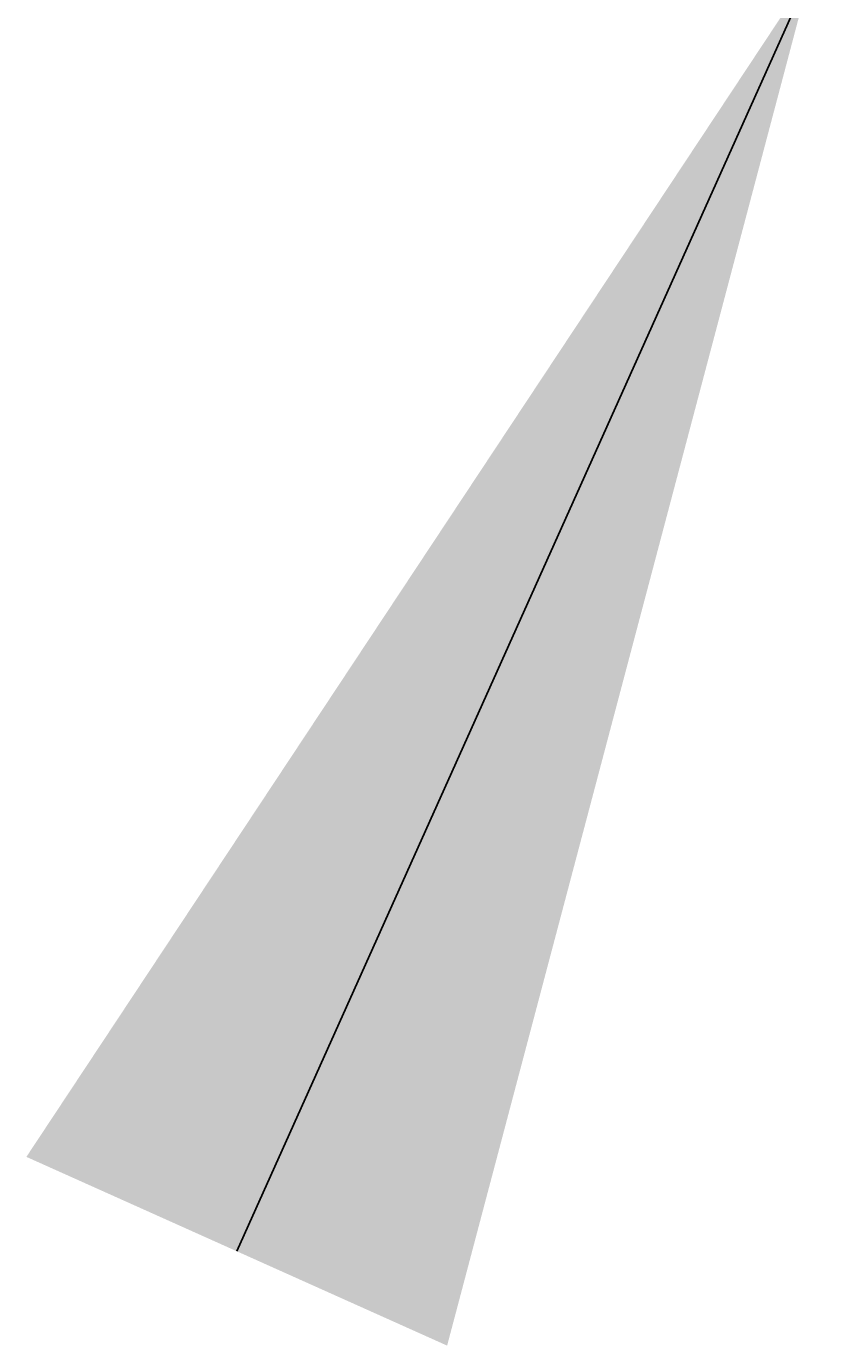
# Model space of a CAD drawing. Units: inches. Extents: x -9413 to 9703, y -9719 to 9096.
# Tile 1 of 1: x -5352 to 276, y -9719 to -311. Entities that reach past the tile are written whole.
import ezdxf
from ezdxf import colors
from ezdxf.entities.mleader import LeaderData, LeaderLine
from ezdxf.math import Vec2, Vec3

# ---------------------------------------------------------------- set-up
doc = ezdxf.new("R2010")
doc.units = ezdxf.units.IN
doc.header["$MEASUREMENT"] = 0
doc.layers.add('M-ANNO-TEXT', color=7, linetype='Continuous', lineweight=18)
doc.styles.get("Standard").update_dxf_attribs({"font": 'arial.ttf'})

msp = doc.modelspace()

# ---------------------------------------------------------------- leaders
at = {"layer": 'M-ANNO-TEXT'}
ml = msp.add_multileader_mtext('Standard', dxfattribs=at)
ml.set_content('Air preheater', color=256)
ml.set_leader_properties()
ml.build(insert=Vec2(0, 0))
ml.multileader.update_dxf_attribs({"dogleg_length": 0.36, "arrow_head_size": 10000, "scale": 10})
ctx = ml.context
ctx.base_point, ctx.scale, ctx.char_height, ctx.arrow_head_size, ctx.landing_gap_size, ctx.plane_origin = Vec3(229.7079293124727, 37.30650895205824), 10, 5.4, 10000, 0.9, Vec3(241.9833706008503, 78.04556948044049)
notes = []
notes.append((ctx, [(1, (1, 1, 0), (223.7048975654645, 37.30650895205824), (1, 0), 6.003031747008185, [(0, [(241.9833706008503, 78.04556948044049)], 0, [])])]))
ctx.mtext.insert, ctx.mtext.flow_direction = Vec3(230.6079293124727, 40.75609967511417), 5
for ctx, leaders in notes:
    for number, flags, end, landing, length, lines in leaders:
        leader = LeaderData()
        leader.index, (leader.has_last_leader_line, leader.has_dogleg_vector, leader.attachment_direction) = number, flags
        leader.last_leader_point, leader.dogleg_vector, leader.dogleg_length = Vec3(end), Vec3(landing), length
        for number, points, colour, breaks in lines:
            line = LeaderLine()
            line.index, line.vertices, line.color, line.breaks = number, Vec3.list(points), colors.encode_raw_color(colour), breaks
            leader.lines.append(line)
        ctx.leaders.append(leader)

doc.saveas('drawing.dxf')
